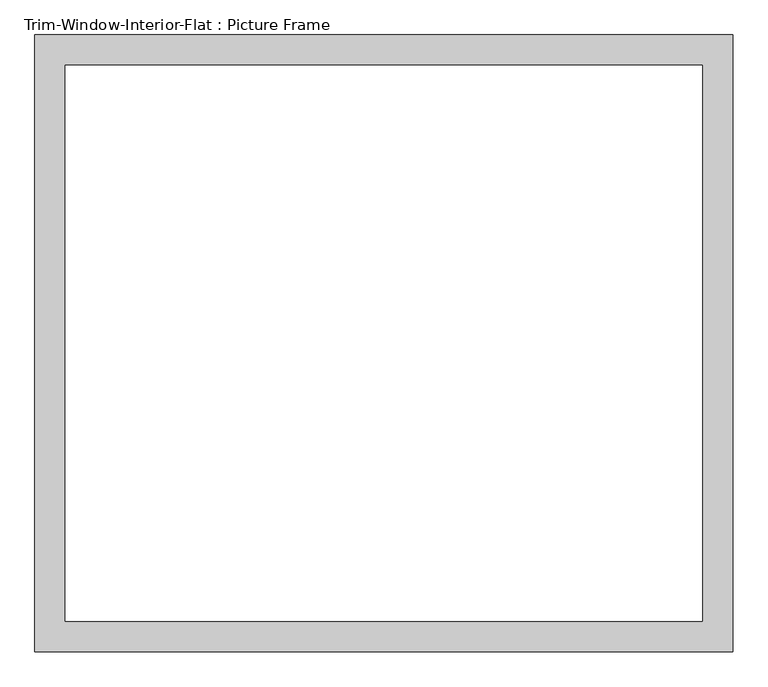
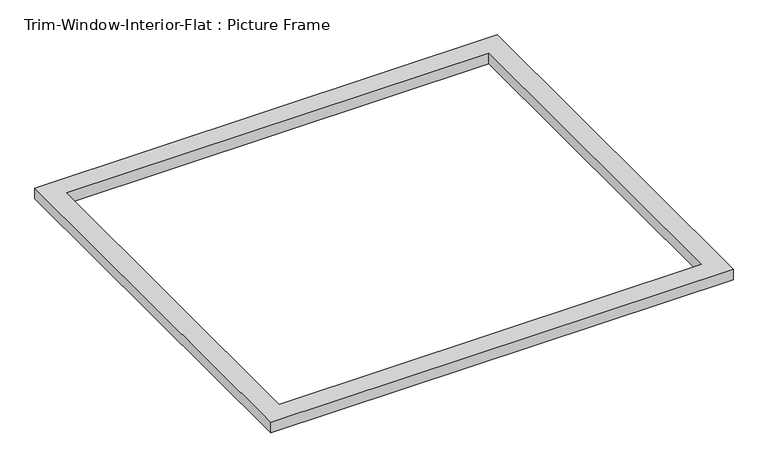
"""IFC4 building model written with IfcOpenShell, lengths in millimetres: proxy geometry, Trim-Window-Interior-Flat : Picture Frame."""

from ifc_helpers import new_model, si_unit, origin, origin_with_axes, place, context, project, spatial, polyline, outline, extrude, source, transform, mapped, element, save


def trim_window_interior_flat_picture_frame_a40cb921(model_context):
    return source(origin(), model_context, "Body", "SweptSolid", [
        extrude(outline(polyline([(654.05, -44.45), (-654.05, -44.45), (-654.05, 1111.25), (654.05, 1111.25), (654.05, -44.45)]), holes=[polyline([(596.9, 12.7), (596.9, 1054.1), (-596.9, 1054.1), (-596.9, 12.7), (596.9, 12.7)])]), origin_with_axes(), (0.0, 0.0, 1.0), 31.75),
    ])


if __name__ == "__main__":
    model = new_model("IFC4")
    model_context = context("Model", 3, world=origin())
    ifc_project = project(units=[si_unit("LENGTHUNIT", "METRE", prefix="MILLI")], contexts=[model_context])
    site = spatial("IfcSite", under=ifc_project)
    building = spatial("IfcBuilding", under=site)
    placement = place(None, origin())
    trim_window_interior_flat_picture_frame_shape = trim_window_interior_flat_picture_frame_a40cb921(model_context)
    element("IfcBuildingElementProxy", 1, Name="Trim-Window-Interior-Flat : Picture Frame", ObjectType="Trim-Window-Interior-Flat : Picture Frame", at=placement, inside=building, context=model_context, shape_type="MappedRepresentation", body=[
        mapped(trim_window_interior_flat_picture_frame_shape, transform((0.0, 0.0, 0.0), x_axis=(1.0, 0.0, 0.0), y_axis=(0.0, 1.0, 0.0), z_axis=(0.0, 0.0, 1.0))),
    ])
    save(model, "model.ifc")

# Revit data of these elements
# Type "Trim-Window-Interior-Flat : Picture Frame"
#   Trim Thickness_Picture Frame = 0' - 1 1/4"
#   Trim Width = 0' - 2 1/4"
#   Trim Thickness_with Sill = 0' - 0 3/4"
#   Sill Thickness = 0' - 1 1/4"
#   Opening Width [instance default] = 2' - 0"
#   Opening Height [instance default] = 3' - 0"
#   Default Elevation = 4' - 0"
#   Sill = no
#   Picture Frame = yes
#   Trim Material [instance default] = none
# Element 1 (IfcBuildingElementProxy, "Trim-Window-Interior-Flat : Picture Frame")
#   Opening Width = 4' - 0"
#   Opening Height = 3' - 6"
#   Trim Material = Wood - Stained
#   Materials on its faces: "Wood - Stained"
# Materials
#   "Wood - Stained": class "Wood", colour RGB 224 178 126, transparency 0, Cost = 0
